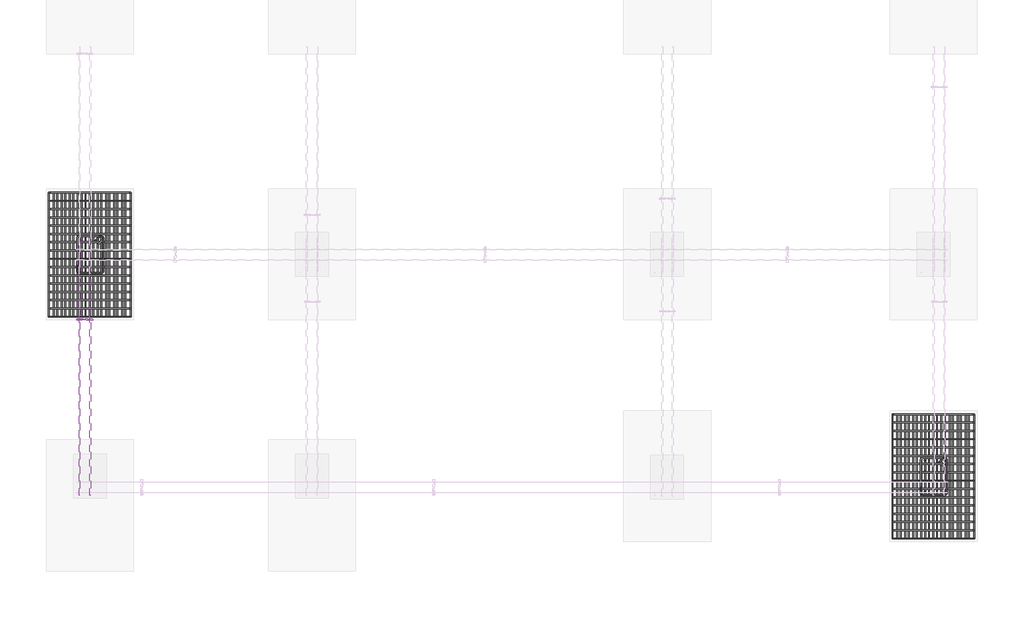
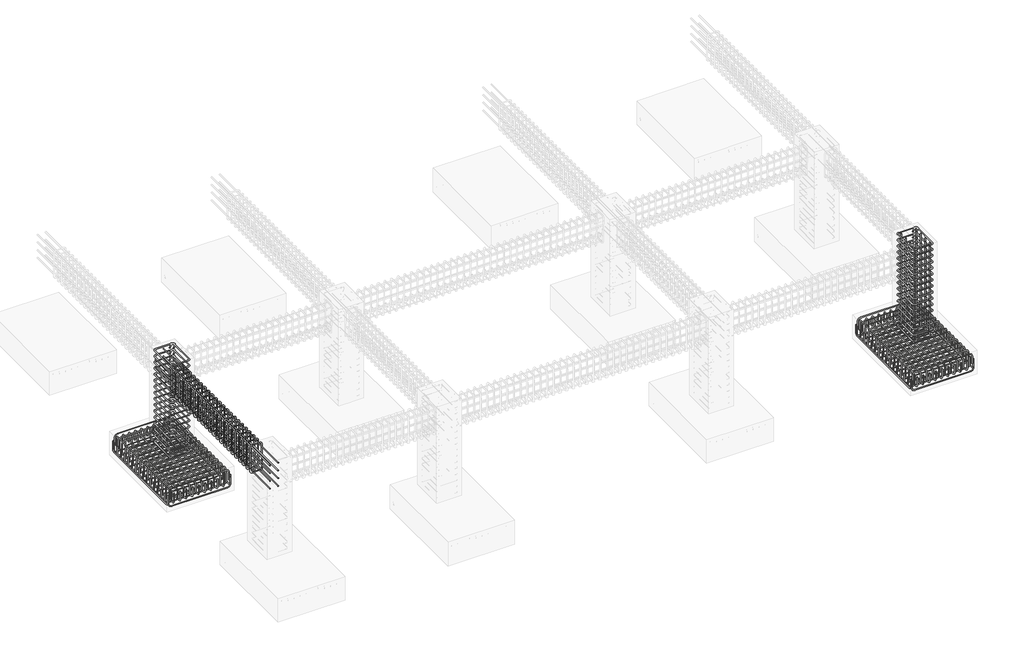
# One storey, part 4 of 16: 15 reinforcing bars.
"""IFC4 building model written with IfcOpenShell, lengths in millimetres."""

from ifc_helpers import new_model, si_unit, point, frame, origin, place, context, project, spatial, polyline, circle_curve, trimmed, segment, composite_curve, source, transform, mapped, element, save
from ifc_brep_helpers import swept_disk

model = new_model("IFC4")

# Units and contexts
model_context = context("Model", 3, world=origin())
ifc_project = project(units=[si_unit("LENGTHUNIT", "METRE", prefix="MILLI")], contexts=[model_context])

# Site, building, storey
site = spatial("IfcSite", under=ifc_project)
building = spatial("IfcBuilding", under=site)
storey = spatial("IfcBuildingStorey", under=building, Elevation=-1828.8)

# Reinforcing bars
placement = place(None, origin())
reinforcing_bar_shape = source(origin(), model_context, "Body", "SolidModel", [
    swept_disk(composite_curve([segment(polyline([(6759.9197974, -311.9348046, -2028.4710597), (6759.9197974, -311.9348046, -2175.7710597)]), True, "CONTINUOUS"), segment(trimmed(circle_curve(frame((6713.5697974, -311.9348046, -2175.7710597), z_axis=(0.0, 1.0, 0.0), x_axis=(46.349999999999454, 0.0, 0.0)), 46.35), [point((6759.9197974, -311.9348046, -2175.7710597))], [point((6713.5697974, -311.9348046, -2222.1210597))], True, "CARTESIAN"), True, "CONTINUOUS"), segment(polyline([(6713.5697974, -311.9348046, -2222.1210597), (5698.9697974, -311.9348046, -2222.1210597)]), True, "CONTINUOUS"), segment(trimmed(circle_curve(frame((5698.9697974, -311.9348046, -2175.7710597), z_axis=(0.0, 1.0, 0.0), x_axis=(0.0, 0.0, -46.34999999999991)), 46.35), [point((5698.9697974, -311.9348046, -2222.1210597))], [point((5652.6197974, -311.9348046, -2175.7710597))], True, "CARTESIAN"), True, "CONTINUOUS"), segment(polyline([(5652.6197974, -311.9348046, -2175.7710597), (5652.6197974, -311.9348046, -2028.4710597)]), True, "CONTINUOUS")], self_intersect=False), 6.35),
])
element("IfcReinforcingBar", 1, at=placement, inside=storey, context=model_context, shape_type="MappedRepresentation", body=[
    mapped(reinforcing_bar_shape, transform((0.0, 0.0, 0.0), x_axis=(1.0, 0.0, 0.0), y_axis=(0.0, 1.0, 0.0), z_axis=(0.0, 0.0, 1.0))),
    mapped(reinforcing_bar_shape, transform((0.0, -113.82, 0.0), x_axis=(1.0, 0.0, 0.0), y_axis=(0.0, 1.0, 0.0), z_axis=(0.0, 0.0, 1.0))),
    mapped(reinforcing_bar_shape, transform((0.0, -227.64, 0.0), x_axis=(1.0, 0.0, 0.0), y_axis=(0.0, 1.0, 0.0), z_axis=(0.0, 0.0, 1.0))),
    mapped(reinforcing_bar_shape, transform((0.0, -341.46, 0.0), x_axis=(1.0, 0.0, 0.0), y_axis=(0.0, 1.0, 0.0), z_axis=(0.0, 0.0, 1.0))),
    mapped(reinforcing_bar_shape, transform((0.0, -455.28, 0.0), x_axis=(1.0, 0.0, 0.0), y_axis=(0.0, 1.0, 0.0), z_axis=(0.0, 0.0, 1.0))),
    mapped(reinforcing_bar_shape, transform((0.0, -569.1, 0.0), x_axis=(1.0, 0.0, 0.0), y_axis=(0.0, 1.0, 0.0), z_axis=(0.0, 0.0, 1.0))),
    mapped(reinforcing_bar_shape, transform((0.0, -682.92, 0.0), x_axis=(1.0, 0.0, 0.0), y_axis=(0.0, 1.0, 0.0), z_axis=(0.0, 0.0, 1.0))),
    mapped(reinforcing_bar_shape, transform((0.0, -796.74, 0.0), x_axis=(1.0, 0.0, 0.0), y_axis=(0.0, 1.0, 0.0), z_axis=(0.0, 0.0, 1.0))),
    mapped(reinforcing_bar_shape, transform((0.0, -910.56, 0.0), x_axis=(1.0, 0.0, 0.0), y_axis=(0.0, 1.0, 0.0), z_axis=(0.0, 0.0, 1.0))),
    mapped(reinforcing_bar_shape, transform((0.0, -1024.38, 0.0), x_axis=(1.0, 0.0, 0.0), y_axis=(0.0, 1.0, 0.0), z_axis=(0.0, 0.0, 1.0))),
    mapped(reinforcing_bar_shape, transform((0.0, -1138.2, 0.0), x_axis=(1.0, 0.0, 0.0), y_axis=(0.0, 1.0, 0.0), z_axis=(0.0, 0.0, 1.0))),
    mapped(reinforcing_bar_shape, transform((0.0, -1252.02, 0.0), x_axis=(1.0, 0.0, 0.0), y_axis=(0.0, 1.0, 0.0), z_axis=(0.0, 0.0, 1.0))),
    mapped(reinforcing_bar_shape, transform((0.0, -1365.84, 0.0), x_axis=(1.0, 0.0, 0.0), y_axis=(0.0, 1.0, 0.0), z_axis=(0.0, 0.0, 1.0))),
    mapped(reinforcing_bar_shape, transform((0.0, -1479.66, 0.0), x_axis=(1.0, 0.0, 0.0), y_axis=(0.0, 1.0, 0.0), z_axis=(0.0, 0.0, 1.0))),
    mapped(reinforcing_bar_shape, transform((0.0, -1593.48, 0.0), x_axis=(1.0, 0.0, 0.0), y_axis=(0.0, 1.0, 0.0), z_axis=(0.0, 0.0, 1.0))),
    mapped(reinforcing_bar_shape, transform((0.0, -1707.3, 0.0), x_axis=(1.0, 0.0, 0.0), y_axis=(0.0, 1.0, 0.0), z_axis=(0.0, 0.0, 1.0))),
])
reinforcing_bar_2_shape = source(origin(), model_context, "Body", "SolidModel", [
    swept_disk(composite_curve([segment(polyline([(5671.0757234, -311.9348046, -2081.4939987), (5671.0757234, -311.9348046, -1934.1939987)]), True, "CONTINUOUS"), segment(trimmed(circle_curve(frame((5717.4257234, -311.9348046, -1934.1939987), z_axis=(0.0, 1.0, 0.0), x_axis=(-46.349999999999454, 0.0, 0.0)), 46.35), [point((5671.0757234, -311.9348046, -1934.1939987))], [point((5717.4257234, -311.9348046, -1887.8439987))], True, "CARTESIAN"), True, "CONTINUOUS"), segment(polyline([(5717.4257234, -311.9348046, -1887.8439987), (6691.1450702, -311.9348046, -1887.8439987)]), True, "CONTINUOUS"), segment(trimmed(circle_curve(frame((6691.1450702, -311.9348046, -1934.1939987), z_axis=(0.0, 1.0, 0.0), x_axis=(0.0, 0.0, 46.350000000000136)), 46.35), [point((6691.1450702, -311.9348046, -1887.8439987))], [point((6737.4950702, -311.9348046, -1934.1939987))], True, "CARTESIAN"), True, "CONTINUOUS"), segment(polyline([(6737.4950702, -311.9348046, -1934.1939987), (6737.4950702, -311.9348046, -2081.4939987)]), True, "CONTINUOUS")], self_intersect=False), 6.35),
])
element("IfcReinforcingBar", 2, at=placement, inside=storey, context=model_context, shape_type="MappedRepresentation", body=[
    mapped(reinforcing_bar_2_shape, transform((0.0, 0.0, 0.0), x_axis=(1.0, 0.0, 0.0), y_axis=(0.0, 1.0, 0.0), z_axis=(0.0, 0.0, 1.0))),
    mapped(reinforcing_bar_2_shape, transform((0.0, -113.82, 0.0), x_axis=(1.0, 0.0, 0.0), y_axis=(0.0, 1.0, 0.0), z_axis=(0.0, 0.0, 1.0))),
    mapped(reinforcing_bar_2_shape, transform((0.0, -227.64, 0.0), x_axis=(1.0, 0.0, 0.0), y_axis=(0.0, 1.0, 0.0), z_axis=(0.0, 0.0, 1.0))),
    mapped(reinforcing_bar_2_shape, transform((0.0, -341.46, 0.0), x_axis=(1.0, 0.0, 0.0), y_axis=(0.0, 1.0, 0.0), z_axis=(0.0, 0.0, 1.0))),
    mapped(reinforcing_bar_2_shape, transform((0.0, -455.28, 0.0), x_axis=(1.0, 0.0, 0.0), y_axis=(0.0, 1.0, 0.0), z_axis=(0.0, 0.0, 1.0))),
    mapped(reinforcing_bar_2_shape, transform((0.0, -569.1, 0.0), x_axis=(1.0, 0.0, 0.0), y_axis=(0.0, 1.0, 0.0), z_axis=(0.0, 0.0, 1.0))),
    mapped(reinforcing_bar_2_shape, transform((0.0, -682.92, 0.0), x_axis=(1.0, 0.0, 0.0), y_axis=(0.0, 1.0, 0.0), z_axis=(0.0, 0.0, 1.0))),
    mapped(reinforcing_bar_2_shape, transform((0.0, -796.74, 0.0), x_axis=(1.0, 0.0, 0.0), y_axis=(0.0, 1.0, 0.0), z_axis=(0.0, 0.0, 1.0))),
    mapped(reinforcing_bar_2_shape, transform((0.0, -910.56, 0.0), x_axis=(1.0, 0.0, 0.0), y_axis=(0.0, 1.0, 0.0), z_axis=(0.0, 0.0, 1.0))),
    mapped(reinforcing_bar_2_shape, transform((0.0, -1024.38, 0.0), x_axis=(1.0, 0.0, 0.0), y_axis=(0.0, 1.0, 0.0), z_axis=(0.0, 0.0, 1.0))),
    mapped(reinforcing_bar_2_shape, transform((0.0, -1138.2, 0.0), x_axis=(1.0, 0.0, 0.0), y_axis=(0.0, 1.0, 0.0), z_axis=(0.0, 0.0, 1.0))),
    mapped(reinforcing_bar_2_shape, transform((0.0, -1252.02, 0.0), x_axis=(1.0, 0.0, 0.0), y_axis=(0.0, 1.0, 0.0), z_axis=(0.0, 0.0, 1.0))),
    mapped(reinforcing_bar_2_shape, transform((0.0, -1365.84, 0.0), x_axis=(1.0, 0.0, 0.0), y_axis=(0.0, 1.0, 0.0), z_axis=(0.0, 0.0, 1.0))),
    mapped(reinforcing_bar_2_shape, transform((0.0, -1479.66, 0.0), x_axis=(1.0, 0.0, 0.0), y_axis=(0.0, 1.0, 0.0), z_axis=(0.0, 0.0, 1.0))),
    mapped(reinforcing_bar_2_shape, transform((0.0, -1593.48, 0.0), x_axis=(1.0, 0.0, 0.0), y_axis=(0.0, 1.0, 0.0), z_axis=(0.0, 0.0, 1.0))),
    mapped(reinforcing_bar_2_shape, transform((0.0, -1707.3, 0.0), x_axis=(1.0, 0.0, 0.0), y_axis=(0.0, 1.0, 0.0), z_axis=(0.0, 0.0, 1.0))),
])
reinforcing_bar_3_shape = source(origin(), model_context, "Body", "SolidModel", [
    swept_disk(composite_curve([segment(polyline([(6687.5434064, -311.9348046, -2112.6585679), (6687.5434064, -311.9348046, -1965.3585679)]), True, "CONTINUOUS"), segment(trimmed(circle_curve(frame((6687.5434064, -358.2848046, -1965.3585679), z_axis=(1.0, 0.0, 0.0), x_axis=(0.0, 46.349999999999966, 0.0)), 46.35), [point((6687.5434064, -311.9348046, -1965.3585679))], [point((6687.5434064, -358.2848046, -1919.0085679))], True, "CARTESIAN"), True, "CONTINUOUS"), segment(polyline([(6687.5434064, -358.2848046, -1919.0085679), (6687.5434064, -1972.8848046, -1919.0085679)]), True, "CONTINUOUS"), segment(trimmed(circle_curve(frame((6687.5434064, -1972.8848046, -1965.3585679), z_axis=(1.0, 0.0, 0.0), x_axis=(0.0, 0.0, 46.350000000000136)), 46.35), [point((6687.5434064, -1972.8848046, -1919.0085679))], [point((6687.5434064, -2019.2348046, -1965.3585679))], True, "CARTESIAN"), True, "CONTINUOUS"), segment(polyline([(6687.5434064, -2019.2348046, -1965.3585679), (6687.5434064, -2019.2348046, -2112.6585679)]), True, "CONTINUOUS")], self_intersect=False), 6.35),
])
element("IfcReinforcingBar", 3, at=placement, inside=storey, context=model_context, shape_type="MappedRepresentation", body=[
    mapped(reinforcing_bar_3_shape, transform((0.0, 0.0, 0.0), x_axis=(1.0, 0.0, 0.0), y_axis=(0.0, 1.0, 0.0), z_axis=(0.0, 0.0, 1.0))),
    mapped(reinforcing_bar_3_shape, transform((-109.2679104, 0.0, 0.0), x_axis=(1.0, 0.0, 0.0), y_axis=(0.0, 1.0, 0.0), z_axis=(0.0, 0.0, 1.0))),
    mapped(reinforcing_bar_3_shape, transform((-218.5358207, 0.0, 0.0), x_axis=(1.0, 0.0, 0.0), y_axis=(0.0, 1.0, 0.0), z_axis=(0.0, 0.0, 1.0))),
    mapped(reinforcing_bar_3_shape, transform((-327.8037311, 0.0, 0.0), x_axis=(1.0, 0.0, 0.0), y_axis=(0.0, 1.0, 0.0), z_axis=(0.0, 0.0, 1.0))),
    mapped(reinforcing_bar_3_shape, transform((-437.0716415, 0.0, 0.0), x_axis=(1.0, 0.0, 0.0), y_axis=(0.0, 1.0, 0.0), z_axis=(0.0, 0.0, 1.0))),
    mapped(reinforcing_bar_3_shape, transform((-546.3395518, 0.0, 0.0), x_axis=(1.0, 0.0, 0.0), y_axis=(0.0, 1.0, 0.0), z_axis=(0.0, 0.0, 1.0))),
    mapped(reinforcing_bar_3_shape, transform((-655.6074622, 0.0, 0.0), x_axis=(1.0, 0.0, 0.0), y_axis=(0.0, 1.0, 0.0), z_axis=(0.0, 0.0, 1.0))),
    mapped(reinforcing_bar_3_shape, transform((-764.8753726, 0.0, 0.0), x_axis=(1.0, 0.0, 0.0), y_axis=(0.0, 1.0, 0.0), z_axis=(0.0, 0.0, 1.0))),
    mapped(reinforcing_bar_3_shape, transform((-874.1432829, 0.0, 0.0), x_axis=(1.0, 0.0, 0.0), y_axis=(0.0, 1.0, 0.0), z_axis=(0.0, 0.0, 1.0))),
    mapped(reinforcing_bar_3_shape, transform((-983.4111933, 0.0, 0.0), x_axis=(1.0, 0.0, 0.0), y_axis=(0.0, 1.0, 0.0), z_axis=(0.0, 0.0, 1.0))),
])
reinforcing_bar_4_shape = source(origin(), model_context, "Body", "SolidModel", [
    swept_disk(composite_curve([segment(polyline([(5639.3657332, -311.9348046, -1996.4434391), (5639.3657332, -311.9348046, -2143.7434391)]), True, "CONTINUOUS"), segment(trimmed(circle_curve(frame((5639.3657332, -358.2848046, -2143.7434391), z_axis=(-1.0, 0.0, 0.0), x_axis=(0.0, 46.349999999999966, 0.0)), 46.35), [point((5639.3657332, -311.9348046, -2143.7434391))], [point((5639.3657332, -358.2848046, -2190.0934391))], True, "CARTESIAN"), True, "CONTINUOUS"), segment(polyline([(5639.3657332, -358.2848046, -2190.0934391), (5639.3657332, -1972.8848046, -2190.0934391)]), True, "CONTINUOUS"), segment(trimmed(circle_curve(frame((5639.3657332, -1972.8848046, -2143.7434391), z_axis=(-1.0, 0.0, 0.0), x_axis=(0.0, 0.0, -46.34999999999991)), 46.35), [point((5639.3657332, -1972.8848046, -2190.0934391))], [point((5639.3657332, -2019.2348046, -2143.7434391))], True, "CARTESIAN"), True, "CONTINUOUS"), segment(polyline([(5639.3657332, -2019.2348046, -2143.7434391), (5639.3657332, -2019.2348046, -1996.4434391)]), True, "CONTINUOUS")], self_intersect=False), 6.35),
])
element("IfcReinforcingBar", 4, at=placement, inside=storey, context=model_context, shape_type="MappedRepresentation", body=[
    mapped(reinforcing_bar_4_shape, transform((0.0, 0.0, 0.0), x_axis=(1.0, 0.0, 0.0), y_axis=(0.0, 1.0, 0.0), z_axis=(0.0, 0.0, 1.0))),
    mapped(reinforcing_bar_4_shape, transform((112.0554064, 0.0, 0.0), x_axis=(1.0, 0.0, 0.0), y_axis=(0.0, 1.0, 0.0), z_axis=(0.0, 0.0, 1.0))),
    mapped(reinforcing_bar_4_shape, transform((224.1108128, 0.0, 0.0), x_axis=(1.0, 0.0, 0.0), y_axis=(0.0, 1.0, 0.0), z_axis=(0.0, 0.0, 1.0))),
    mapped(reinforcing_bar_4_shape, transform((336.1662192, 0.0, 0.0), x_axis=(1.0, 0.0, 0.0), y_axis=(0.0, 1.0, 0.0), z_axis=(0.0, 0.0, 1.0))),
    mapped(reinforcing_bar_4_shape, transform((448.2216256, 0.0, 0.0), x_axis=(1.0, 0.0, 0.0), y_axis=(0.0, 1.0, 0.0), z_axis=(0.0, 0.0, 1.0))),
    mapped(reinforcing_bar_4_shape, transform((560.2770321, 0.0, 0.0), x_axis=(1.0, 0.0, 0.0), y_axis=(0.0, 1.0, 0.0), z_axis=(0.0, 0.0, 1.0))),
    mapped(reinforcing_bar_4_shape, transform((672.3324385, 0.0, 0.0), x_axis=(1.0, 0.0, 0.0), y_axis=(0.0, 1.0, 0.0), z_axis=(0.0, 0.0, 1.0))),
    mapped(reinforcing_bar_4_shape, transform((784.3878449, 0.0, 0.0), x_axis=(1.0, 0.0, 0.0), y_axis=(0.0, 1.0, 0.0), z_axis=(0.0, 0.0, 1.0))),
    mapped(reinforcing_bar_4_shape, transform((896.4432513, 0.0, 0.0), x_axis=(1.0, 0.0, 0.0), y_axis=(0.0, 1.0, 0.0), z_axis=(0.0, 0.0, 1.0))),
    mapped(reinforcing_bar_4_shape, transform((1008.4986577, 0.0, 0.0), x_axis=(1.0, 0.0, 0.0), y_axis=(0.0, 1.0, 0.0), z_axis=(0.0, 0.0, 1.0))),
    mapped(reinforcing_bar_4_shape, transform((1120.5540641, 0.0, 0.0), x_axis=(1.0, 0.0, 0.0), y_axis=(0.0, 1.0, 0.0), z_axis=(0.0, 0.0, 1.0))),
])
reinforcing_bar_5_shape = source(origin(), model_context, "Body", "SolidModel", [
    swept_disk(composite_curve([segment(polyline([(-4822.4802026, 2736.0651954, -2028.4710597), (-4822.4802026, 2736.0651954, -2175.7710597)]), True, "CONTINUOUS"), segment(trimmed(circle_curve(frame((-4868.8302026, 2736.0651954, -2175.7710597), z_axis=(0.0, 1.0, 0.0), x_axis=(46.350000000000364, 0.0, 0.0)), 46.35), [point((-4822.4802026, 2736.0651954, -2175.7710597))], [point((-4868.8302026, 2736.0651954, -2222.1210597))], True, "CARTESIAN"), True, "CONTINUOUS"), segment(polyline([(-4868.8302026, 2736.0651954, -2222.1210597), (-5883.4302026, 2736.0651954, -2222.1210597)]), True, "CONTINUOUS"), segment(trimmed(circle_curve(frame((-5883.4302026, 2736.0651954, -2175.7710597), z_axis=(0.0, 1.0, 0.0), x_axis=(0.0, 0.0, -46.34999999999991)), 46.35), [point((-5883.4302026, 2736.0651954, -2222.1210597))], [point((-5929.7802026, 2736.0651954, -2175.7710597))], True, "CARTESIAN"), True, "CONTINUOUS"), segment(polyline([(-5929.7802026, 2736.0651954, -2175.7710597), (-5929.7802026, 2736.0651954, -2028.4710597)]), True, "CONTINUOUS")], self_intersect=False), 6.35),
])
element("IfcReinforcingBar", 5, at=placement, inside=storey, context=model_context, shape_type="MappedRepresentation", body=[
    mapped(reinforcing_bar_5_shape, transform((0.0, 0.0, 0.0), x_axis=(1.0, 0.0, 0.0), y_axis=(0.0, 1.0, 0.0), z_axis=(0.0, 0.0, 1.0))),
    mapped(reinforcing_bar_5_shape, transform((0.0, -113.82, 0.0), x_axis=(1.0, 0.0, 0.0), y_axis=(0.0, 1.0, 0.0), z_axis=(0.0, 0.0, 1.0))),
    mapped(reinforcing_bar_5_shape, transform((0.0, -227.64, 0.0), x_axis=(1.0, 0.0, 0.0), y_axis=(0.0, 1.0, 0.0), z_axis=(0.0, 0.0, 1.0))),
    mapped(reinforcing_bar_5_shape, transform((0.0, -341.46, 0.0), x_axis=(1.0, 0.0, 0.0), y_axis=(0.0, 1.0, 0.0), z_axis=(0.0, 0.0, 1.0))),
    mapped(reinforcing_bar_5_shape, transform((0.0, -455.28, 0.0), x_axis=(1.0, 0.0, 0.0), y_axis=(0.0, 1.0, 0.0), z_axis=(0.0, 0.0, 1.0))),
    mapped(reinforcing_bar_5_shape, transform((0.0, -569.1, 0.0), x_axis=(1.0, 0.0, 0.0), y_axis=(0.0, 1.0, 0.0), z_axis=(0.0, 0.0, 1.0))),
    mapped(reinforcing_bar_5_shape, transform((0.0, -682.92, 0.0), x_axis=(1.0, 0.0, 0.0), y_axis=(0.0, 1.0, 0.0), z_axis=(0.0, 0.0, 1.0))),
    mapped(reinforcing_bar_5_shape, transform((0.0, -796.74, 0.0), x_axis=(1.0, 0.0, 0.0), y_axis=(0.0, 1.0, 0.0), z_axis=(0.0, 0.0, 1.0))),
    mapped(reinforcing_bar_5_shape, transform((0.0, -910.56, 0.0), x_axis=(1.0, 0.0, 0.0), y_axis=(0.0, 1.0, 0.0), z_axis=(0.0, 0.0, 1.0))),
    mapped(reinforcing_bar_5_shape, transform((0.0, -1024.38, 0.0), x_axis=(1.0, 0.0, 0.0), y_axis=(0.0, 1.0, 0.0), z_axis=(0.0, 0.0, 1.0))),
    mapped(reinforcing_bar_5_shape, transform((0.0, -1138.2, 0.0), x_axis=(1.0, 0.0, 0.0), y_axis=(0.0, 1.0, 0.0), z_axis=(0.0, 0.0, 1.0))),
    mapped(reinforcing_bar_5_shape, transform((0.0, -1252.02, 0.0), x_axis=(1.0, 0.0, 0.0), y_axis=(0.0, 1.0, 0.0), z_axis=(0.0, 0.0, 1.0))),
    mapped(reinforcing_bar_5_shape, transform((0.0, -1365.84, 0.0), x_axis=(1.0, 0.0, 0.0), y_axis=(0.0, 1.0, 0.0), z_axis=(0.0, 0.0, 1.0))),
    mapped(reinforcing_bar_5_shape, transform((0.0, -1479.66, 0.0), x_axis=(1.0, 0.0, 0.0), y_axis=(0.0, 1.0, 0.0), z_axis=(0.0, 0.0, 1.0))),
    mapped(reinforcing_bar_5_shape, transform((0.0, -1593.48, 0.0), x_axis=(1.0, 0.0, 0.0), y_axis=(0.0, 1.0, 0.0), z_axis=(0.0, 0.0, 1.0))),
    mapped(reinforcing_bar_5_shape, transform((0.0, -1707.3, 0.0), x_axis=(1.0, 0.0, 0.0), y_axis=(0.0, 1.0, 0.0), z_axis=(0.0, 0.0, 1.0))),
])
reinforcing_bar_6_shape = source(origin(), model_context, "Body", "SolidModel", [
    swept_disk(composite_curve([segment(polyline([(-5911.3242766, 2736.0651954, -2081.4939987), (-5911.3242766, 2736.0651954, -1934.1939987)]), True, "CONTINUOUS"), segment(trimmed(circle_curve(frame((-5864.9742766, 2736.0651954, -1934.1939987), z_axis=(0.0, 1.0, 0.0), x_axis=(-46.350000000000364, 0.0, 0.0)), 46.35), [point((-5911.3242766, 2736.0651954, -1934.1939987))], [point((-5864.9742766, 2736.0651954, -1887.8439987))], True, "CARTESIAN"), True, "CONTINUOUS"), segment(polyline([(-5864.9742766, 2736.0651954, -1887.8439987), (-4891.2549298, 2736.0651954, -1887.8439987)]), True, "CONTINUOUS"), segment(trimmed(circle_curve(frame((-4891.2549298, 2736.0651954, -1934.1939987), z_axis=(0.0, 1.0, 0.0), x_axis=(0.0, 0.0, 46.350000000000136)), 46.35), [point((-4891.2549298, 2736.0651954, -1887.8439987))], [point((-4844.9049298, 2736.0651954, -1934.1939987))], True, "CARTESIAN"), True, "CONTINUOUS"), segment(polyline([(-4844.9049298, 2736.0651954, -1934.1939987), (-4844.9049298, 2736.0651954, -2081.4939987)]), True, "CONTINUOUS")], self_intersect=False), 6.35),
])
element("IfcReinforcingBar", 6, at=placement, inside=storey, context=model_context, shape_type="MappedRepresentation", body=[
    mapped(reinforcing_bar_6_shape, transform((0.0, 0.0, 0.0), x_axis=(1.0, 0.0, 0.0), y_axis=(0.0, 1.0, 0.0), z_axis=(0.0, 0.0, 1.0))),
    mapped(reinforcing_bar_6_shape, transform((0.0, -113.82, 0.0), x_axis=(1.0, 0.0, 0.0), y_axis=(0.0, 1.0, 0.0), z_axis=(0.0, 0.0, 1.0))),
    mapped(reinforcing_bar_6_shape, transform((0.0, -227.64, 0.0), x_axis=(1.0, 0.0, 0.0), y_axis=(0.0, 1.0, 0.0), z_axis=(0.0, 0.0, 1.0))),
    mapped(reinforcing_bar_6_shape, transform((0.0, -341.46, 0.0), x_axis=(1.0, 0.0, 0.0), y_axis=(0.0, 1.0, 0.0), z_axis=(0.0, 0.0, 1.0))),
    mapped(reinforcing_bar_6_shape, transform((0.0, -455.28, 0.0), x_axis=(1.0, 0.0, 0.0), y_axis=(0.0, 1.0, 0.0), z_axis=(0.0, 0.0, 1.0))),
    mapped(reinforcing_bar_6_shape, transform((0.0, -569.1, 0.0), x_axis=(1.0, 0.0, 0.0), y_axis=(0.0, 1.0, 0.0), z_axis=(0.0, 0.0, 1.0))),
    mapped(reinforcing_bar_6_shape, transform((0.0, -682.92, 0.0), x_axis=(1.0, 0.0, 0.0), y_axis=(0.0, 1.0, 0.0), z_axis=(0.0, 0.0, 1.0))),
    mapped(reinforcing_bar_6_shape, transform((0.0, -796.74, 0.0), x_axis=(1.0, 0.0, 0.0), y_axis=(0.0, 1.0, 0.0), z_axis=(0.0, 0.0, 1.0))),
    mapped(reinforcing_bar_6_shape, transform((0.0, -910.56, 0.0), x_axis=(1.0, 0.0, 0.0), y_axis=(0.0, 1.0, 0.0), z_axis=(0.0, 0.0, 1.0))),
    mapped(reinforcing_bar_6_shape, transform((0.0, -1024.38, 0.0), x_axis=(1.0, 0.0, 0.0), y_axis=(0.0, 1.0, 0.0), z_axis=(0.0, 0.0, 1.0))),
    mapped(reinforcing_bar_6_shape, transform((0.0, -1138.2, 0.0), x_axis=(1.0, 0.0, 0.0), y_axis=(0.0, 1.0, 0.0), z_axis=(0.0, 0.0, 1.0))),
    mapped(reinforcing_bar_6_shape, transform((0.0, -1252.02, 0.0), x_axis=(1.0, 0.0, 0.0), y_axis=(0.0, 1.0, 0.0), z_axis=(0.0, 0.0, 1.0))),
    mapped(reinforcing_bar_6_shape, transform((0.0, -1365.84, 0.0), x_axis=(1.0, 0.0, 0.0), y_axis=(0.0, 1.0, 0.0), z_axis=(0.0, 0.0, 1.0))),
    mapped(reinforcing_bar_6_shape, transform((0.0, -1479.66, 0.0), x_axis=(1.0, 0.0, 0.0), y_axis=(0.0, 1.0, 0.0), z_axis=(0.0, 0.0, 1.0))),
    mapped(reinforcing_bar_6_shape, transform((0.0, -1593.48, 0.0), x_axis=(1.0, 0.0, 0.0), y_axis=(0.0, 1.0, 0.0), z_axis=(0.0, 0.0, 1.0))),
    mapped(reinforcing_bar_6_shape, transform((0.0, -1707.3, 0.0), x_axis=(1.0, 0.0, 0.0), y_axis=(0.0, 1.0, 0.0), z_axis=(0.0, 0.0, 1.0))),
])
reinforcing_bar_7_shape = source(origin(), model_context, "Body", "SolidModel", [
    swept_disk(composite_curve([segment(polyline([(-4894.8565936, 2736.0651954, -2112.6585679), (-4894.8565936, 2736.0651954, -1965.3585679)]), True, "CONTINUOUS"), segment(trimmed(circle_curve(frame((-4894.8565936, 2689.7151954, -1965.3585679), z_axis=(1.0, 0.0, 0.0), x_axis=(0.0, 46.34999999999991, 0.0)), 46.35), [point((-4894.8565936, 2736.0651954, -1965.3585679))], [point((-4894.8565936, 2689.7151954, -1919.0085679))], True, "CARTESIAN"), True, "CONTINUOUS"), segment(polyline([(-4894.8565936, 2689.7151954, -1919.0085679), (-4894.8565936, 1075.1151954, -1919.0085679)]), True, "CONTINUOUS"), segment(trimmed(circle_curve(frame((-4894.8565936, 1075.1151954, -1965.3585679), z_axis=(1.0, 0.0, 0.0), x_axis=(0.0, 0.0, 46.350000000000136)), 46.35), [point((-4894.8565936, 1075.1151954, -1919.0085679))], [point((-4894.8565936, 1028.7651954, -1965.3585679))], True, "CARTESIAN"), True, "CONTINUOUS"), segment(polyline([(-4894.8565936, 1028.7651954, -1965.3585679), (-4894.8565936, 1028.7651954, -2112.6585679)]), True, "CONTINUOUS")], self_intersect=False), 6.35),
])
element("IfcReinforcingBar", 7, at=placement, inside=storey, context=model_context, shape_type="MappedRepresentation", body=[
    mapped(reinforcing_bar_7_shape, transform((0.0, 0.0, 0.0), x_axis=(1.0, 0.0, 0.0), y_axis=(0.0, 1.0, 0.0), z_axis=(0.0, 0.0, 1.0))),
    mapped(reinforcing_bar_7_shape, transform((-109.2679104, 0.0, 0.0), x_axis=(1.0, 0.0, 0.0), y_axis=(0.0, 1.0, 0.0), z_axis=(0.0, 0.0, 1.0))),
    mapped(reinforcing_bar_7_shape, transform((-218.5358207, 0.0, 0.0), x_axis=(1.0, 0.0, 0.0), y_axis=(0.0, 1.0, 0.0), z_axis=(0.0, 0.0, 1.0))),
    mapped(reinforcing_bar_7_shape, transform((-327.8037311, 0.0, 0.0), x_axis=(1.0, 0.0, 0.0), y_axis=(0.0, 1.0, 0.0), z_axis=(0.0, 0.0, 1.0))),
    mapped(reinforcing_bar_7_shape, transform((-437.0716415, 0.0, 0.0), x_axis=(1.0, 0.0, 0.0), y_axis=(0.0, 1.0, 0.0), z_axis=(0.0, 0.0, 1.0))),
    mapped(reinforcing_bar_7_shape, transform((-546.3395518, 0.0, 0.0), x_axis=(1.0, 0.0, 0.0), y_axis=(0.0, 1.0, 0.0), z_axis=(0.0, 0.0, 1.0))),
    mapped(reinforcing_bar_7_shape, transform((-655.6074622, 0.0, 0.0), x_axis=(1.0, 0.0, 0.0), y_axis=(0.0, 1.0, 0.0), z_axis=(0.0, 0.0, 1.0))),
    mapped(reinforcing_bar_7_shape, transform((-764.8753726, 0.0, 0.0), x_axis=(1.0, 0.0, 0.0), y_axis=(0.0, 1.0, 0.0), z_axis=(0.0, 0.0, 1.0))),
    mapped(reinforcing_bar_7_shape, transform((-874.1432829, 0.0, 0.0), x_axis=(1.0, 0.0, 0.0), y_axis=(0.0, 1.0, 0.0), z_axis=(0.0, 0.0, 1.0))),
    mapped(reinforcing_bar_7_shape, transform((-983.4111933, 0.0, 0.0), x_axis=(1.0, 0.0, 0.0), y_axis=(0.0, 1.0, 0.0), z_axis=(0.0, 0.0, 1.0))),
])
reinforcing_bar_8_shape = source(origin(), model_context, "Body", "SolidModel", [
    swept_disk(composite_curve([segment(polyline([(-5943.0342668, 2736.0651954, -1996.4434391), (-5943.0342668, 2736.0651954, -2143.7434391)]), True, "CONTINUOUS"), segment(trimmed(circle_curve(frame((-5943.0342668, 2689.7151954, -2143.7434391), z_axis=(-1.0, 0.0, 0.0), x_axis=(0.0, 46.34999999999991, 0.0)), 46.35), [point((-5943.0342668, 2736.0651954, -2143.7434391))], [point((-5943.0342668, 2689.7151954, -2190.0934391))], True, "CARTESIAN"), True, "CONTINUOUS"), segment(polyline([(-5943.0342668, 2689.7151954, -2190.0934391), (-5943.0342668, 1075.1151954, -2190.0934391)]), True, "CONTINUOUS"), segment(trimmed(circle_curve(frame((-5943.0342668, 1075.1151954, -2143.7434391), z_axis=(-1.0, 0.0, 0.0), x_axis=(0.0, 0.0, -46.34999999999991)), 46.35), [point((-5943.0342668, 1075.1151954, -2190.0934391))], [point((-5943.0342668, 1028.7651954, -2143.7434391))], True, "CARTESIAN"), True, "CONTINUOUS"), segment(polyline([(-5943.0342668, 1028.7651954, -2143.7434391), (-5943.0342668, 1028.7651954, -1996.4434391)]), True, "CONTINUOUS")], self_intersect=False), 6.35),
])
element("IfcReinforcingBar", 8, at=placement, inside=storey, context=model_context, shape_type="MappedRepresentation", body=[
    mapped(reinforcing_bar_8_shape, transform((0.0, 0.0, 0.0), x_axis=(1.0, 0.0, 0.0), y_axis=(0.0, 1.0, 0.0), z_axis=(0.0, 0.0, 1.0))),
    mapped(reinforcing_bar_8_shape, transform((112.0554064, 0.0, 0.0), x_axis=(1.0, 0.0, 0.0), y_axis=(0.0, 1.0, 0.0), z_axis=(0.0, 0.0, 1.0))),
    mapped(reinforcing_bar_8_shape, transform((224.1108128, 0.0, 0.0), x_axis=(1.0, 0.0, 0.0), y_axis=(0.0, 1.0, 0.0), z_axis=(0.0, 0.0, 1.0))),
    mapped(reinforcing_bar_8_shape, transform((336.1662192, 0.0, 0.0), x_axis=(1.0, 0.0, 0.0), y_axis=(0.0, 1.0, 0.0), z_axis=(0.0, 0.0, 1.0))),
    mapped(reinforcing_bar_8_shape, transform((448.2216256, 0.0, 0.0), x_axis=(1.0, 0.0, 0.0), y_axis=(0.0, 1.0, 0.0), z_axis=(0.0, 0.0, 1.0))),
    mapped(reinforcing_bar_8_shape, transform((560.2770321, 0.0, 0.0), x_axis=(1.0, 0.0, 0.0), y_axis=(0.0, 1.0, 0.0), z_axis=(0.0, 0.0, 1.0))),
    mapped(reinforcing_bar_8_shape, transform((672.3324385, 0.0, 0.0), x_axis=(1.0, 0.0, 0.0), y_axis=(0.0, 1.0, 0.0), z_axis=(0.0, 0.0, 1.0))),
    mapped(reinforcing_bar_8_shape, transform((784.3878449, 0.0, 0.0), x_axis=(1.0, 0.0, 0.0), y_axis=(0.0, 1.0, 0.0), z_axis=(0.0, 0.0, 1.0))),
    mapped(reinforcing_bar_8_shape, transform((896.4432513, 0.0, 0.0), x_axis=(1.0, 0.0, 0.0), y_axis=(0.0, 1.0, 0.0), z_axis=(0.0, 0.0, 1.0))),
    mapped(reinforcing_bar_8_shape, transform((1008.4986577, 0.0, 0.0), x_axis=(1.0, 0.0, 0.0), y_axis=(0.0, 1.0, 0.0), z_axis=(0.0, 0.0, 1.0))),
    mapped(reinforcing_bar_8_shape, transform((1120.5540641, 0.0, 0.0), x_axis=(1.0, 0.0, 0.0), y_axis=(0.0, 1.0, 0.0), z_axis=(0.0, 0.0, 1.0))),
])
reinforcing_bar_9_shape = source(origin(), model_context, "Body", "SolidModel", [
    swept_disk(composite_curve([segment(polyline([(6275.6584368, -976.86057, -46.35), (6331.4019998, -921.117007, -46.35)]), True, "CONTINUOUS"), segment(trimmed(circle_curve(frame((6353.5697974, -943.2848046, -46.35), z_axis=(0.0, 0.0, -1.0), x_axis=(-22.167797600000085, 22.167797600000085, 0.0)), 31.35), [point((6331.4019998, -921.117007, -46.35))], [point((6384.9197974, -943.2848046, -46.35))], True, "CARTESIAN"), True, "CONTINUOUS"), segment(polyline([(6384.9197974, -943.2848046, -46.35), (6384.9197974, -1387.8848046, -46.35)]), True, "CONTINUOUS"), segment(trimmed(circle_curve(frame((6353.5697974, -1387.8848046, -46.35), z_axis=(0.0, 0.0, -1.0), x_axis=(31.349999999999454, 0.0, 0.0)), 31.35), [point((6384.9197974, -1387.8848046, -46.35))], [point((6353.5697974, -1419.2348046, -46.35))], True, "CARTESIAN"), True, "CONTINUOUS"), segment(polyline([(6353.5697974, -1419.2348046, -46.35), (6058.9697974, -1419.2348046, -46.35)]), True, "CONTINUOUS"), segment(trimmed(circle_curve(frame((6058.9697974, -1387.8946239, -45.5654144), z_axis=(0.0, 0.025026655153786343, -0.9996867842138424), x_axis=(0.0, -31.34018070000002, -0.7845855999999998)), 31.35), [point((6058.9697974, -1419.2348046, -46.35))], [point((6027.6197974, -1387.8946239, -45.5654144))], True, "CARTESIAN"), True, "CONTINUOUS"), segment(polyline([(6027.6197974, -1387.8946239, -45.5654144), (6027.6197974, -943.2749853, -34.4345856)]), True, "CONTINUOUS"), segment(trimmed(circle_curve(frame((6058.9697974, -943.2749853, -34.4345856), z_axis=(0.0, 0.025026655153786343, -0.9996867842138424), x_axis=(-31.350000000000364, 0.0, 0.0)), 31.35), [point((6027.6197974, -943.2749853, -34.4345856))], [point((6058.9697974, -911.9348046, -33.65))], True, "CARTESIAN"), True, "CONTINUOUS"), segment(polyline([(6058.9697974, -911.9348046, -33.65), (6353.5697974, -911.9348046, -33.65)]), True, "CONTINUOUS"), segment(trimmed(circle_curve(frame((6353.5697974, -943.2848046, -33.65), z_axis=(0.0, 0.0, -1.0), x_axis=(0.0, 31.350000000000023, 0.0)), 31.35), [point((6353.5697974, -911.9348046, -33.65))], [point((6375.737595, -965.4526022, -33.65))], True, "CARTESIAN"), True, "CONTINUOUS"), segment(polyline([(6375.737595, -965.4526022, -33.65), (6319.994032, -1021.1961652, -33.65)]), True, "CONTINUOUS")], self_intersect=False), 6.35),
])
element("IfcReinforcingBar", 9, at=placement, inside=storey, context=model_context, shape_type="MappedRepresentation", body=[
    mapped(reinforcing_bar_9_shape, transform((0.0, 0.0, 0.0), x_axis=(1.0, 0.0, 0.0), y_axis=(0.0, 1.0, 0.0), z_axis=(0.0, 0.0, 1.0))),
    mapped(reinforcing_bar_9_shape, transform((0.0, 0.0, -115.74), x_axis=(1.0, 0.0, 0.0), y_axis=(0.0, 1.0, 0.0), z_axis=(0.0, 0.0, 1.0))),
    mapped(reinforcing_bar_9_shape, transform((0.0, 0.0, -231.48), x_axis=(1.0, 0.0, 0.0), y_axis=(0.0, 1.0, 0.0), z_axis=(0.0, 0.0, 1.0))),
    mapped(reinforcing_bar_9_shape, transform((0.0, 0.0, -347.22), x_axis=(1.0, 0.0, 0.0), y_axis=(0.0, 1.0, 0.0), z_axis=(0.0, 0.0, 1.0))),
    mapped(reinforcing_bar_9_shape, transform((0.0, 0.0, -462.96), x_axis=(1.0, 0.0, 0.0), y_axis=(0.0, 1.0, 0.0), z_axis=(0.0, 0.0, 1.0))),
    mapped(reinforcing_bar_9_shape, transform((0.0, 0.0, -578.7), x_axis=(1.0, 0.0, 0.0), y_axis=(0.0, 1.0, 0.0), z_axis=(0.0, 0.0, 1.0))),
    mapped(reinforcing_bar_9_shape, transform((0.0, 0.0, -694.44), x_axis=(1.0, 0.0, 0.0), y_axis=(0.0, 1.0, 0.0), z_axis=(0.0, 0.0, 1.0))),
    mapped(reinforcing_bar_9_shape, transform((0.0, 0.0, -810.18), x_axis=(1.0, 0.0, 0.0), y_axis=(0.0, 1.0, 0.0), z_axis=(0.0, 0.0, 1.0))),
    mapped(reinforcing_bar_9_shape, transform((0.0, 0.0, -925.92), x_axis=(1.0, 0.0, 0.0), y_axis=(0.0, 1.0, 0.0), z_axis=(0.0, 0.0, 1.0))),
    mapped(reinforcing_bar_9_shape, transform((0.0, 0.0, -1041.66), x_axis=(1.0, 0.0, 0.0), y_axis=(0.0, 1.0, 0.0), z_axis=(0.0, 0.0, 1.0))),
    mapped(reinforcing_bar_9_shape, transform((0.0, 0.0, -1157.4), x_axis=(1.0, 0.0, 0.0), y_axis=(0.0, 1.0, 0.0), z_axis=(0.0, 0.0, 1.0))),
    mapped(reinforcing_bar_9_shape, transform((0.0, 0.0, -1273.14), x_axis=(1.0, 0.0, 0.0), y_axis=(0.0, 1.0, 0.0), z_axis=(0.0, 0.0, 1.0))),
    mapped(reinforcing_bar_9_shape, transform((0.0, 0.0, -1388.88), x_axis=(1.0, 0.0, 0.0), y_axis=(0.0, 1.0, 0.0), z_axis=(0.0, 0.0, 1.0))),
    mapped(reinforcing_bar_9_shape, transform((0.0, 0.0, -1504.62), x_axis=(1.0, 0.0, 0.0), y_axis=(0.0, 1.0, 0.0), z_axis=(0.0, 0.0, 1.0))),
    mapped(reinforcing_bar_9_shape, transform((0.0, 0.0, -1620.36), x_axis=(1.0, 0.0, 0.0), y_axis=(0.0, 1.0, 0.0), z_axis=(0.0, 0.0, 1.0))),
    mapped(reinforcing_bar_9_shape, transform((0.0, 0.0, -1736.1), x_axis=(1.0, 0.0, 0.0), y_axis=(0.0, 1.0, 0.0), z_axis=(0.0, 0.0, 1.0))),
])
reinforcing_bar_10_shape = source(origin(), model_context, "Body", "SolidModel", [
    swept_disk(composite_curve([segment(polyline([(6350.3822559, -950.0668285, -40.0), (6350.3822559, -950.0668285, -1788.8)]), True, "CONTINUOUS")], self_intersect=False), 6.35),
])
element("IfcReinforcingBar", 10, at=placement, inside=storey, context=model_context, shape_type="MappedRepresentation", body=[
    mapped(reinforcing_bar_10_shape, transform((0.0, 0.0, 0.0), x_axis=(1.0, 0.0, 0.0), y_axis=(0.0, 1.0, 0.0), z_axis=(0.0, 0.0, 1.0))),
    mapped(reinforcing_bar_10_shape, transform((0.0, -141.8865927, 0.0), x_axis=(1.0, 0.0, 0.0), y_axis=(0.0, 1.0, 0.0), z_axis=(0.0, 0.0, 1.0))),
    mapped(reinforcing_bar_10_shape, transform((0.0, -283.7731853, 0.0), x_axis=(1.0, 0.0, 0.0), y_axis=(0.0, 1.0, 0.0), z_axis=(0.0, 0.0, 1.0))),
    mapped(reinforcing_bar_10_shape, transform((0.0, -425.659778, 0.0), x_axis=(1.0, 0.0, 0.0), y_axis=(0.0, 1.0, 0.0), z_axis=(0.0, 0.0, 1.0))),
])
reinforcing_bar_11_shape = source(origin(), model_context, "Body", "SolidModel", [
    swept_disk(composite_curve([segment(polyline([(6082.1573388, -950.0668285, -40.0), (6082.1573388, -950.0668285, -1788.8)]), True, "CONTINUOUS")], self_intersect=False), 6.35),
])
element("IfcReinforcingBar", 11, at=placement, inside=storey, context=model_context, shape_type="MappedRepresentation", body=[
    mapped(reinforcing_bar_11_shape, transform((0.0, 0.0, 0.0), x_axis=(1.0, 0.0, 0.0), y_axis=(0.0, 1.0, 0.0), z_axis=(0.0, 0.0, 1.0))),
    mapped(reinforcing_bar_11_shape, transform((0.0, -141.8865927, 0.0), x_axis=(1.0, 0.0, 0.0), y_axis=(0.0, 1.0, 0.0), z_axis=(0.0, 0.0, 1.0))),
    mapped(reinforcing_bar_11_shape, transform((0.0, -283.7731853, 0.0), x_axis=(1.0, 0.0, 0.0), y_axis=(0.0, 1.0, 0.0), z_axis=(0.0, 0.0, 1.0))),
    mapped(reinforcing_bar_11_shape, transform((0.0, -425.659778, 0.0), x_axis=(1.0, 0.0, 0.0), y_axis=(0.0, 1.0, 0.0), z_axis=(0.0, 0.0, 1.0))),
])
reinforcing_bar_12_shape = source(origin(), model_context, "Body", "SolidModel", [
    swept_disk(composite_curve([segment(polyline([(-5306.7415632, 2071.13943, -46.35), (-5250.9980002, 2126.882993, -46.35)]), True, "CONTINUOUS"), segment(trimmed(circle_curve(frame((-5228.8302026, 2104.7151954, -46.35), z_axis=(0.0, 0.0, -1.0), x_axis=(-22.167797600000085, 22.167797600000085, 0.0)), 31.35), [point((-5250.9980002, 2126.882993, -46.35))], [point((-5197.4802026, 2104.7151954, -46.35))], True, "CARTESIAN"), True, "CONTINUOUS"), segment(polyline([(-5197.4802026, 2104.7151954, -46.35), (-5197.4802026, 1660.1151954, -46.35)]), True, "CONTINUOUS"), segment(trimmed(circle_curve(frame((-5228.8302026, 1660.1151954, -46.35), z_axis=(0.0, 0.0, -1.0), x_axis=(31.350000000000364, 0.0, 0.0)), 31.35), [point((-5197.4802026, 1660.1151954, -46.35))], [point((-5228.8302026, 1628.7651954, -46.35))], True, "CARTESIAN"), True, "CONTINUOUS"), segment(polyline([(-5228.8302026, 1628.7651954, -46.35), (-5523.4302026, 1628.7651954, -46.35)]), True, "CONTINUOUS"), segment(trimmed(circle_curve(frame((-5523.4302026, 1660.1053761, -45.5654144), z_axis=(0.0, 0.025026655153786343, -0.9996867842138424), x_axis=(0.0, -31.34018070000002, -0.7845855999999998)), 31.35), [point((-5523.4302026, 1628.7651954, -46.35))], [point((-5554.7802026, 1660.1053761, -45.5654144))], True, "CARTESIAN"), True, "CONTINUOUS"), segment(polyline([(-5554.7802026, 1660.1053761, -45.5654144), (-5554.7802026, 2104.7250147, -34.4345856)]), True, "CONTINUOUS"), segment(trimmed(circle_curve(frame((-5523.4302026, 2104.7250147, -34.4345856), z_axis=(0.0, 0.025026655153786343, -0.9996867842138424), x_axis=(-31.350000000000364, 0.0, 0.0)), 31.35), [point((-5554.7802026, 2104.7250147, -34.4345856))], [point((-5523.4302026, 2136.0651954, -33.65))], True, "CARTESIAN"), True, "CONTINUOUS"), segment(polyline([(-5523.4302026, 2136.0651954, -33.65), (-5228.8302026, 2136.0651954, -33.65)]), True, "CONTINUOUS"), segment(trimmed(circle_curve(frame((-5228.8302026, 2104.7151954, -33.65), z_axis=(0.0, 0.0, -1.0), x_axis=(0.0, 31.34999999999991, 0.0)), 31.35), [point((-5228.8302026, 2136.0651954, -33.65))], [point((-5206.662405, 2082.5473978, -33.65))], True, "CARTESIAN"), True, "CONTINUOUS"), segment(polyline([(-5206.662405, 2082.5473978, -33.65), (-5262.405968, 2026.8038348, -33.65)]), True, "CONTINUOUS")], self_intersect=False), 6.35),
])
element("IfcReinforcingBar", 12, at=placement, inside=storey, context=model_context, shape_type="MappedRepresentation", body=[
    mapped(reinforcing_bar_12_shape, transform((0.0, 0.0, 0.0), x_axis=(1.0, 0.0, 0.0), y_axis=(0.0, 1.0, 0.0), z_axis=(0.0, 0.0, 1.0))),
    mapped(reinforcing_bar_12_shape, transform((0.0, 0.0, -115.74), x_axis=(1.0, 0.0, 0.0), y_axis=(0.0, 1.0, 0.0), z_axis=(0.0, 0.0, 1.0))),
    mapped(reinforcing_bar_12_shape, transform((0.0, 0.0, -231.48), x_axis=(1.0, 0.0, 0.0), y_axis=(0.0, 1.0, 0.0), z_axis=(0.0, 0.0, 1.0))),
    mapped(reinforcing_bar_12_shape, transform((0.0, 0.0, -347.22), x_axis=(1.0, 0.0, 0.0), y_axis=(0.0, 1.0, 0.0), z_axis=(0.0, 0.0, 1.0))),
    mapped(reinforcing_bar_12_shape, transform((0.0, 0.0, -462.96), x_axis=(1.0, 0.0, 0.0), y_axis=(0.0, 1.0, 0.0), z_axis=(0.0, 0.0, 1.0))),
    mapped(reinforcing_bar_12_shape, transform((0.0, 0.0, -578.7), x_axis=(1.0, 0.0, 0.0), y_axis=(0.0, 1.0, 0.0), z_axis=(0.0, 0.0, 1.0))),
    mapped(reinforcing_bar_12_shape, transform((0.0, 0.0, -694.44), x_axis=(1.0, 0.0, 0.0), y_axis=(0.0, 1.0, 0.0), z_axis=(0.0, 0.0, 1.0))),
    mapped(reinforcing_bar_12_shape, transform((0.0, 0.0, -810.18), x_axis=(1.0, 0.0, 0.0), y_axis=(0.0, 1.0, 0.0), z_axis=(0.0, 0.0, 1.0))),
    mapped(reinforcing_bar_12_shape, transform((0.0, 0.0, -925.92), x_axis=(1.0, 0.0, 0.0), y_axis=(0.0, 1.0, 0.0), z_axis=(0.0, 0.0, 1.0))),
    mapped(reinforcing_bar_12_shape, transform((0.0, 0.0, -1041.66), x_axis=(1.0, 0.0, 0.0), y_axis=(0.0, 1.0, 0.0), z_axis=(0.0, 0.0, 1.0))),
    mapped(reinforcing_bar_12_shape, transform((0.0, 0.0, -1157.4), x_axis=(1.0, 0.0, 0.0), y_axis=(0.0, 1.0, 0.0), z_axis=(0.0, 0.0, 1.0))),
    mapped(reinforcing_bar_12_shape, transform((0.0, 0.0, -1273.14), x_axis=(1.0, 0.0, 0.0), y_axis=(0.0, 1.0, 0.0), z_axis=(0.0, 0.0, 1.0))),
    mapped(reinforcing_bar_12_shape, transform((0.0, 0.0, -1388.88), x_axis=(1.0, 0.0, 0.0), y_axis=(0.0, 1.0, 0.0), z_axis=(0.0, 0.0, 1.0))),
    mapped(reinforcing_bar_12_shape, transform((0.0, 0.0, -1504.62), x_axis=(1.0, 0.0, 0.0), y_axis=(0.0, 1.0, 0.0), z_axis=(0.0, 0.0, 1.0))),
    mapped(reinforcing_bar_12_shape, transform((0.0, 0.0, -1620.36), x_axis=(1.0, 0.0, 0.0), y_axis=(0.0, 1.0, 0.0), z_axis=(0.0, 0.0, 1.0))),
    mapped(reinforcing_bar_12_shape, transform((0.0, 0.0, -1736.1), x_axis=(1.0, 0.0, 0.0), y_axis=(0.0, 1.0, 0.0), z_axis=(0.0, 0.0, 1.0))),
])
reinforcing_bar_13_shape = source(origin(), model_context, "Body", "SolidModel", [
    swept_disk(composite_curve([segment(polyline([(-5445.5188421, -859.2348046, -488.7242346), (-5501.262405, -859.2348046, -544.4677976)]), True, "CONTINUOUS"), segment(trimmed(circle_curve(frame((-5523.4302026, -859.2348046, -522.3), z_axis=(0.0, 1.0, 0.0), x_axis=(22.167797599999176, 0.0, -22.167797600000085)), 31.35), [point((-5501.262405, -859.2348046, -544.4677976))], [point((-5554.7802026, -859.2348046, -522.3))], True, "CARTESIAN"), True, "CONTINUOUS"), segment(polyline([(-5554.7802026, -859.2348046, -522.3), (-5554.7802026, -859.2348046, -77.7)]), True, "CONTINUOUS"), segment(trimmed(circle_curve(frame((-5523.4302026, -859.2348046, -77.7), z_axis=(0.0, 1.0, 0.0), x_axis=(-31.350000000000364, 0.0, 0.0)), 31.35), [point((-5554.7802026, -859.2348046, -77.7))], [point((-5523.4302026, -859.2348046, -46.35))], True, "CARTESIAN"), True, "CONTINUOUS"), segment(polyline([(-5523.4302026, -859.2348046, -46.35), (-5378.8302026, -859.2348046, -46.35)]), True, "CONTINUOUS"), segment(trimmed(circle_curve(frame((-5378.8302026, -860.0193903, -77.6901807), z_axis=(0.0, 0.9996867842138424, -0.025026655153786322), x_axis=(0.0, 0.7845857000000933, 31.340180699999998)), 31.35), [point((-5378.8302026, -859.2348046, -46.35))], [point((-5347.4802026, -860.0193903, -77.6901807))], True, "CARTESIAN"), True, "CONTINUOUS"), segment(polyline([(-5347.4802026, -860.0193903, -77.6901807), (-5347.4802026, -871.150219, -522.3098193)]), True, "CONTINUOUS"), segment(trimmed(circle_curve(frame((-5378.8302026, -871.150219, -522.3098193), z_axis=(0.0, 0.9996867842138424, -0.025026655153786322), x_axis=(31.350000000000364, 0.0, 0.0)), 31.35), [point((-5347.4802026, -871.150219, -522.3098193))], [point((-5378.8302026, -871.9348046, -553.65))], True, "CARTESIAN"), True, "CONTINUOUS"), segment(polyline([(-5378.8302026, -871.9348046, -553.65), (-5523.4302026, -871.9348046, -553.65)]), True, "CONTINUOUS"), segment(trimmed(circle_curve(frame((-5523.4302026, -871.9348046, -522.3), z_axis=(0.0, 1.0, 0.0), x_axis=(0.0, 0.0, -31.350000000000023)), 31.35), [point((-5523.4302026, -871.9348046, -553.65))], [point((-5545.5980002, -871.9348046, -500.1322024))], True, "CARTESIAN"), True, "CONTINUOUS"), segment(polyline([(-5545.5980002, -871.9348046, -500.1322024), (-5489.8544373, -871.9348046, -444.3886395)]), True, "CONTINUOUS")], self_intersect=False), 6.35),
])
element("IfcReinforcingBar", 13, at=placement, inside=storey, context=model_context, shape_type="MappedRepresentation", body=[
    mapped(reinforcing_bar_13_shape, transform((0.0, 0.0, 0.0), x_axis=(1.0, 0.0, 0.0), y_axis=(0.0, 1.0, 0.0), z_axis=(0.0, 0.0, 1.0))),
    mapped(reinforcing_bar_13_shape, transform((0.0, 115.9666667, 0.0), x_axis=(1.0, 0.0, 0.0), y_axis=(0.0, 1.0, 0.0), z_axis=(0.0, 0.0, 1.0))),
    mapped(reinforcing_bar_13_shape, transform((0.0, 231.9333333, 0.0), x_axis=(1.0, 0.0, 0.0), y_axis=(0.0, 1.0, 0.0), z_axis=(0.0, 0.0, 1.0))),
    mapped(reinforcing_bar_13_shape, transform((0.0, 347.9, 0.0), x_axis=(1.0, 0.0, 0.0), y_axis=(0.0, 1.0, 0.0), z_axis=(0.0, 0.0, 1.0))),
    mapped(reinforcing_bar_13_shape, transform((0.0, 463.8666667, 0.0), x_axis=(1.0, 0.0, 0.0), y_axis=(0.0, 1.0, 0.0), z_axis=(0.0, 0.0, 1.0))),
    mapped(reinforcing_bar_13_shape, transform((0.0, 579.8333333, 0.0), x_axis=(1.0, 0.0, 0.0), y_axis=(0.0, 1.0, 0.0), z_axis=(0.0, 0.0, 1.0))),
    mapped(reinforcing_bar_13_shape, transform((0.0, 695.8, 0.0), x_axis=(1.0, 0.0, 0.0), y_axis=(0.0, 1.0, 0.0), z_axis=(0.0, 0.0, 1.0))),
    mapped(reinforcing_bar_13_shape, transform((0.0, 811.7666667, 0.0), x_axis=(1.0, 0.0, 0.0), y_axis=(0.0, 1.0, 0.0), z_axis=(0.0, 0.0, 1.0))),
    mapped(reinforcing_bar_13_shape, transform((0.0, 927.7333333, 0.0), x_axis=(1.0, 0.0, 0.0), y_axis=(0.0, 1.0, 0.0), z_axis=(0.0, 0.0, 1.0))),
    mapped(reinforcing_bar_13_shape, transform((0.0, 1043.7, 0.0), x_axis=(1.0, 0.0, 0.0), y_axis=(0.0, 1.0, 0.0), z_axis=(0.0, 0.0, 1.0))),
    mapped(reinforcing_bar_13_shape, transform((0.0, 1159.6666667, 0.0), x_axis=(1.0, 0.0, 0.0), y_axis=(0.0, 1.0, 0.0), z_axis=(0.0, 0.0, 1.0))),
    mapped(reinforcing_bar_13_shape, transform((0.0, 1275.6333333, 0.0), x_axis=(1.0, 0.0, 0.0), y_axis=(0.0, 1.0, 0.0), z_axis=(0.0, 0.0, 1.0))),
    mapped(reinforcing_bar_13_shape, transform((0.0, 1391.6, 0.0), x_axis=(1.0, 0.0, 0.0), y_axis=(0.0, 1.0, 0.0), z_axis=(0.0, 0.0, 1.0))),
    mapped(reinforcing_bar_13_shape, transform((0.0, 1507.5666667, 0.0), x_axis=(1.0, 0.0, 0.0), y_axis=(0.0, 1.0, 0.0), z_axis=(0.0, 0.0, 1.0))),
    mapped(reinforcing_bar_13_shape, transform((0.0, 1623.5333333, 0.0), x_axis=(1.0, 0.0, 0.0), y_axis=(0.0, 1.0, 0.0), z_axis=(0.0, 0.0, 1.0))),
    mapped(reinforcing_bar_13_shape, transform((0.0, 1739.5, 0.0), x_axis=(1.0, 0.0, 0.0), y_axis=(0.0, 1.0, 0.0), z_axis=(0.0, 0.0, 1.0))),
    mapped(reinforcing_bar_13_shape, transform((0.0, 1855.4666667, 0.0), x_axis=(1.0, 0.0, 0.0), y_axis=(0.0, 1.0, 0.0), z_axis=(0.0, 0.0, 1.0))),
    mapped(reinforcing_bar_13_shape, transform((0.0, 1971.4333333, 0.0), x_axis=(1.0, 0.0, 0.0), y_axis=(0.0, 1.0, 0.0), z_axis=(0.0, 0.0, 1.0))),
    mapped(reinforcing_bar_13_shape, transform((0.0, 2087.4, 0.0), x_axis=(1.0, 0.0, 0.0), y_axis=(0.0, 1.0, 0.0), z_axis=(0.0, 0.0, 1.0))),
    mapped(reinforcing_bar_13_shape, transform((0.0, 2203.3666667, 0.0), x_axis=(1.0, 0.0, 0.0), y_axis=(0.0, 1.0, 0.0), z_axis=(0.0, 0.0, 1.0))),
    mapped(reinforcing_bar_13_shape, transform((0.0, 2319.3333333, 0.0), x_axis=(1.0, 0.0, 0.0), y_axis=(0.0, 1.0, 0.0), z_axis=(0.0, 0.0, 1.0))),
    mapped(reinforcing_bar_13_shape, transform((0.0, 2435.3, 0.0), x_axis=(1.0, 0.0, 0.0), y_axis=(0.0, 1.0, 0.0), z_axis=(0.0, 0.0, 1.0))),
])
reinforcing_bar_14_shape = source(origin(), model_context, "Body", "SolidModel", [
    swept_disk(composite_curve([segment(polyline([(-5523.4302026, -1425.5848046, -524.4645649), (-5523.4302026, 2142.4151954, -524.4645649)]), True, "CONTINUOUS")], self_intersect=False), 6.35),
])
element("IfcReinforcingBar", 14, at=placement, inside=storey, context=model_context, shape_type="MappedRepresentation", body=[
    mapped(reinforcing_bar_14_shape, transform((0.0, 0.0, 0.0), x_axis=(1.0, 0.0, 0.0), y_axis=(0.0, 1.0, 0.0), z_axis=(0.0, 0.0, 1.0))),
    mapped(reinforcing_bar_14_shape, transform((0.0, 0.0, 146.3763852), x_axis=(1.0, 0.0, 0.0), y_axis=(0.0, 1.0, 0.0), z_axis=(0.0, 0.0, 1.0))),
    mapped(reinforcing_bar_14_shape, transform((0.0, 0.0, 292.7527704), x_axis=(1.0, 0.0, 0.0), y_axis=(0.0, 1.0, 0.0), z_axis=(0.0, 0.0, 1.0))),
    mapped(reinforcing_bar_14_shape, transform((0.0, 0.0, 439.1291556), x_axis=(1.0, 0.0, 0.0), y_axis=(0.0, 1.0, 0.0), z_axis=(0.0, 0.0, 1.0))),
])
reinforcing_bar_15_shape = source(origin(), model_context, "Body", "SolidModel", [
    swept_disk(composite_curve([segment(polyline([(-5378.8302026, -1425.5848046, -524.4645649), (-5378.8302026, 2142.4151954, -524.4645649)]), True, "CONTINUOUS")], self_intersect=False), 6.35),
])
element("IfcReinforcingBar", 15, at=placement, inside=storey, context=model_context, shape_type="MappedRepresentation", body=[
    mapped(reinforcing_bar_15_shape, transform((0.0, 0.0, 0.0), x_axis=(1.0, 0.0, 0.0), y_axis=(0.0, 1.0, 0.0), z_axis=(0.0, 0.0, 1.0))),
    mapped(reinforcing_bar_15_shape, transform((0.0, 0.0, 146.3763852), x_axis=(1.0, 0.0, 0.0), y_axis=(0.0, 1.0, 0.0), z_axis=(0.0, 0.0, 1.0))),
    mapped(reinforcing_bar_15_shape, transform((0.0, 0.0, 292.7527704), x_axis=(1.0, 0.0, 0.0), y_axis=(0.0, 1.0, 0.0), z_axis=(0.0, 0.0, 1.0))),
    mapped(reinforcing_bar_15_shape, transform((0.0, 0.0, 439.1291556), x_axis=(1.0, 0.0, 0.0), y_axis=(0.0, 1.0, 0.0), z_axis=(0.0, 0.0, 1.0))),
])

save(model, "model.ifc")

# Revit data of these elements
# Elements 1, 2, 3, 4, 5, 6, 7, 8, 9, 10, 11, 12, 13, 14, 15 (IfcReinforcingBar)
#   Phase Created = New Construction
